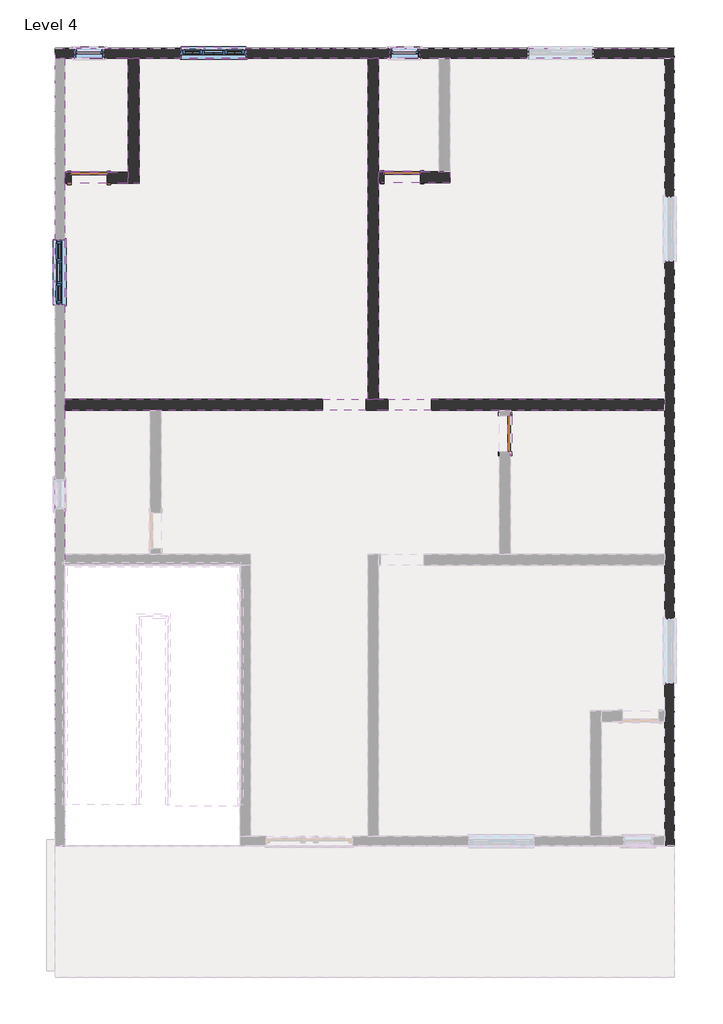
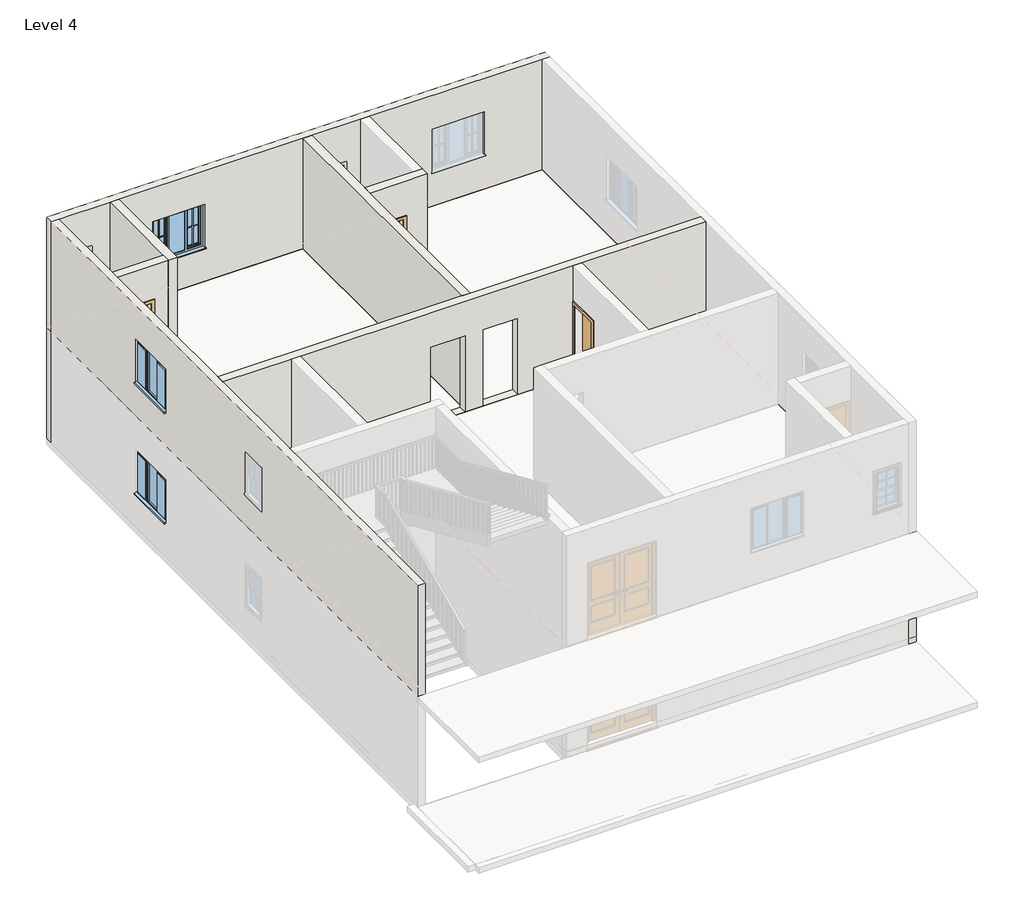
# One storey, part 2 of 5: 20 walls, 12 windows, 9 doors.
"""IFC4 building model written with IfcOpenShell, lengths in millimetres."""

from ifc_helpers import new_model, si_unit, frame, origin, place, context, project, spatial, polyline, outline, extrude, faceted_brep, transform, mapped, element, save
from components import door_85036156, window_679d2811, windows_tpl_w_glazing_cross_bars_1360x1210mm_0306471f

model = new_model("IFC4")

# Units and contexts
model_context = context("Model", 3, world=origin())
ifc_project = project(units=[si_unit("LENGTHUNIT", "METRE", prefix="MILLI")], contexts=[model_context])

# Site, building, storey
site = spatial("IfcSite", under=ifc_project)
building = spatial("IfcBuilding", under=site)
storey = spatial("IfcBuildingStorey", under=building, Name="Level 4", Elevation=9144.0)

# Doors
placement = place(None, origin())
door_shape = door_85036156(model_context)
element("IfcDoor", 1, ObjectType="Single-Flush : 30\" x 80\"", at=placement, inside=storey, context=model_context, shape_type="MappedRepresentation", body=[
    mapped(door_shape, transform((-7046.4415084, 6189.6935985, 9144.0), x_axis=(-1.0, 0.0, 0.0), y_axis=(0.0, -1.0, 0.0), z_axis=(0.0, 0.0, 1.0))),
])
element("IfcDoor", 2, ObjectType="Single-Flush : 30\" x 80\"", at=placement, inside=storey, context=model_context, shape_type="MappedRepresentation", body=[
    mapped(door_shape, transform((-467.8415084, 6203.2000968, 9144.0), x_axis=(-1.0, 0.0, 0.0), y_axis=(0.0, -1.0, 0.0), z_axis=(0.0, 0.0, 1.0))),
])
element("IfcDoor", 3, ObjectType="Single-Flush : 30\" x 80\"", at=placement, inside=storey, context=model_context, shape_type="MappedRepresentation", body=[
    mapped(door_shape, transform((1691.1584916, 817.5935985, 9144.0), x_axis=(0.0, 1.0, 0.0), y_axis=(-1.0, 0.0, 0.0), z_axis=(0.0, 0.0, 1.0))),
])
element("IfcDoor", 4, ObjectType="Single-Flush : 30\" x 80\"", at=placement, inside=storey, context=model_context, shape_type="MappedRepresentation", body=[
    mapped(door_shape, transform((-7046.4415084, 6189.6935985, 9144.0), x_axis=(-1.0, 0.0, 0.0), y_axis=(0.0, -1.0, 0.0), z_axis=(0.0, 0.0, 1.0))),
])
element("IfcDoor", 5, ObjectType="Single-Flush : 30\" x 80\"", at=placement, inside=storey, context=model_context, shape_type="MappedRepresentation", body=[
    mapped(door_shape, transform((-467.8415084, 6203.2000968, 9144.0), x_axis=(-1.0, 0.0, 0.0), y_axis=(0.0, -1.0, 0.0), z_axis=(0.0, 0.0, 1.0))),
])
element("IfcDoor", 6, ObjectType="Single-Flush : 30\" x 80\"", at=placement, inside=storey, context=model_context, shape_type="MappedRepresentation", body=[
    mapped(door_shape, transform((1691.1584916, 817.5935985, 9144.0), x_axis=(0.0, 1.0, 0.0), y_axis=(-1.0, 0.0, 0.0), z_axis=(0.0, 0.0, 1.0))),
])
element("IfcDoor", 7, ObjectType="Single-Flush : 30\" x 80\"", at=placement, inside=storey, context=model_context, shape_type="MappedRepresentation", body=[
    mapped(door_shape, transform((-7046.4415084, 6189.6935985, 12192.0), x_axis=(-1.0, 0.0, 0.0), y_axis=(0.0, -1.0, 0.0), z_axis=(0.0, 0.0, 1.0))),
])
element("IfcDoor", 8, ObjectType="Single-Flush : 30\" x 80\"", at=placement, inside=storey, context=model_context, shape_type="MappedRepresentation", body=[
    mapped(door_shape, transform((-467.8415084, 6203.2000968, 12192.0), x_axis=(-1.0, 0.0, 0.0), y_axis=(0.0, -1.0, 0.0), z_axis=(0.0, 0.0, 1.0))),
])
element("IfcDoor", 9, ObjectType="Single-Flush : 30\" x 80\"", at=placement, inside=storey, context=model_context, shape_type="MappedRepresentation", body=[
    mapped(door_shape, transform((1691.1584916, 817.5935985, 12192.0), x_axis=(0.0, 1.0, 0.0), y_axis=(-1.0, 0.0, 0.0), z_axis=(0.0, 0.0, 1.0))),
])

# Walls
element("IfcWall", 10, ObjectType="Generic - 4.5\"", at=placement, inside=storey, context=model_context, shape_type="Brep", body=[
    faceted_brep([(-1232.0415084, 1312.8935985, 11254.0), (-1232.0415084, 1312.8935985, 9144.0), (-770.4415084, 1312.8935985, 9144.0), (-770.4415084, 1312.8935985, 11254.0), (139.5584916, 1312.8935985, 11254.0), (139.5584916, 1312.8935985, 9144.0), (1576.8584916, 1312.8935985, 9144.0), (1805.4584916, 1312.8935985, 9144.0), (5043.9584916, 1312.8935985, 9144.0), (5043.9584916, 1312.8935985, 12192.0), (1805.4584916, 1312.8935985, 12192.0), (1576.8584916, 1312.8935985, 12192.0), (-5535.1415084, 1312.8935985, 12192.0), (-5763.7415084, 1312.8935985, 12192.0), (-7554.4415084, 1312.8935985, 12192.0), (-7554.4415084, 1312.8935985, 9144.0), (-5763.7415084, 1312.8935985, 9144.0), (-5535.1415084, 1312.8935985, 9144.0), (-2142.0415084, 1312.8935985, 9144.0), (-2142.0415084, 1312.8935985, 11254.0), (-770.4415084, 1541.4935985, 9144.0), (-963.1415084, 1541.4935985, 9144.0), (-1191.7415084, 1541.4935985, 9144.0), (-1232.0415084, 1541.4935985, 9144.0), (-1232.0415084, 1541.4935985, 11254.0), (-2142.0415084, 1541.4935985, 11254.0), (-2142.0415084, 1541.4935985, 9144.0), (-7554.4415084, 1541.4935985, 9144.0), (-7554.4415084, 1541.4935985, 12192.0), (-1191.7415084, 1541.4935985, 12192.0), (-963.1415084, 1541.4935985, 12192.0), (5043.9584916, 1541.4935985, 12192.0), (5043.9584916, 1541.4935985, 9144.0), (139.5584916, 1541.4935985, 9144.0), (139.5584916, 1541.4935985, 11254.0), (-770.4415084, 1541.4935985, 11254.0)], [[[0, 1, 2, 3, 4, 5, 6, 7, 8, 9, 10, 11, 12, 13, 14, 15, 16, 17, 18, 19]], [[20, 21, 22, 23, 24, 25, 26, 27, 28, 29, 30, 31, 32, 33, 34, 35]], [[33, 32, 8, 7, 6, 5]], [[2, 1, 23, 22, 21, 20]], [[18, 17, 16, 15, 27, 26]], [[14, 13, 12, 11, 10, 9, 31, 30, 29, 28]], [[9, 8, 32, 31]], [[15, 14, 28, 27]], [[5, 4, 34, 33]], [[3, 2, 20, 35]], [[4, 3, 35, 34]], [[26, 25, 19, 18]], [[24, 23, 1, 0]], [[25, 24, 0, 19]]]),
])
element("IfcWall", 11, ObjectType="Generic - 4.5\"", at=placement, inside=storey, context=model_context, shape_type="Brep", body=[
    faceted_brep([(-1191.7415084, 8704.2935985, 9144.0), (-1191.7415084, 1541.4935985, 9144.0), (-1191.7415084, 1541.4935985, 12192.0), (-1191.7415084, 8704.2935985, 12192.0), (-963.1415084, 8704.2935985, 9144.0), (-963.1415084, 8704.2935985, 12192.0), (-963.1415084, 6317.5000968, 12192.0), (-963.1415084, 6088.9000968, 12192.0), (-963.1415084, 1541.4935985, 12192.0), (-963.1415084, 1541.4935985, 9144.0), (-963.1415084, 6088.9000968, 9144.0), (-963.1415084, 6317.5000968, 9144.0)], [[[0, 1, 2, 3]], [[4, 5, 6, 7, 8, 9, 10, 11]], [[1, 0, 4, 11, 10, 9]], [[3, 2, 8, 7, 6, 5]], [[0, 3, 5, 4]], [[2, 1, 9, 8]]]),
])
element("IfcWall", 12, ObjectType="Generic - 4.5\"", at=placement, inside=storey, context=model_context, shape_type="Brep", body=[
    faceted_brep([(-6220.9415084, 8704.2935985, 9144.0), (-6220.9415084, 6303.9935985, 9144.0), (-6220.9415084, 6075.3935985, 9144.0), (-6220.9415084, 6075.3935985, 12192.0), (-6220.9415084, 6303.9935985, 12192.0), (-6220.9415084, 8704.2935985, 12192.0), (-5992.3415084, 8704.2935985, 9144.0), (-5992.3415084, 8704.2935985, 12192.0), (-5992.3415084, 6075.3935985, 12192.0), (-5992.3415084, 6075.3935985, 9144.0)], [[[0, 1, 2, 3, 4, 5]], [[6, 7, 8, 9]], [[2, 1, 0, 6, 9]], [[5, 4, 3, 8, 7]], [[0, 5, 7, 6]], [[3, 2, 9, 8]]]),
])
element("IfcWall", 13, ObjectType="Generic - 4.5\"", at=placement, inside=storey, context=model_context, shape_type="SweptSolid", body=[
    extrude(outline(polyline([(9144.0, -7554.4415084), (9144.0, -7427.4415084), (11176.0, -7427.4415084), (11176.0, -6665.4415084), (9144.0, -6665.4415084), (9144.0, -6220.9415084), (12192.0, -6220.9415084), (12192.0, -7554.4415084), (9144.0, -7554.4415084)])), frame((0.0, 6075.3935985, 0.0), z_axis=(0.0, 1.0, 0.0), x_axis=(0.0, 0.0, 1.0)), (0.0, 0.0, 1.0), 228.6),
])
element("IfcWall", 14, ObjectType="Generic - 4.5\"", at=placement, inside=storey, context=model_context, shape_type="Brep", body=[
    faceted_brep([(-963.1415084, 6088.9000968, 9144.0), (-848.8415084, 6088.9000968, 9144.0), (-848.8415084, 6088.9000968, 11176.0), (-86.8415084, 6088.9000968, 11176.0), (-86.8415084, 6088.9000968, 9144.0), (535.4584916, 6088.9000968, 9144.0), (535.4584916, 6088.9000968, 12192.0), (-963.1415084, 6088.9000968, 12192.0), (-848.8415084, 6317.5000968, 11176.0), (-848.8415084, 6317.5000968, 9144.0), (-963.1415084, 6317.5000968, 9144.0), (-963.1415084, 6317.5000968, 12192.0), (306.8584916, 6317.5000968, 12192.0), (535.4584916, 6317.5000968, 12192.0), (535.4584916, 6317.5000968, 9144.0), (306.8584916, 6317.5000968, 9144.0), (-86.8415084, 6317.5000968, 9144.0), (-86.8415084, 6317.5000968, 11176.0)], [[[0, 1, 2, 3, 4, 5, 6, 7]], [[8, 9, 10, 11, 12, 13, 14, 15, 16, 17]], [[10, 9, 1, 0]], [[16, 15, 14, 5, 4]], [[7, 6, 13, 12, 11]], [[0, 7, 11, 10]], [[6, 5, 14, 13]], [[2, 1, 9, 8]], [[3, 2, 8, 17]], [[4, 3, 17, 16]]]),
])
element("IfcWall", 15, ObjectType="Generic - 4.5\"", at=placement, inside=storey, context=model_context, shape_type="Brep", body=[
    faceted_brep([(-1232.0415084, 1312.8935985, 11254.0), (-1232.0415084, 1312.8935985, 9144.0), (-770.4415084, 1312.8935985, 9144.0), (-770.4415084, 1312.8935985, 11254.0), (139.5584916, 1312.8935985, 11254.0), (139.5584916, 1312.8935985, 9144.0), (1576.8584916, 1312.8935985, 9144.0), (1805.4584916, 1312.8935985, 9144.0), (5043.9584916, 1312.8935985, 9144.0), (5043.9584916, 1312.8935985, 12192.0), (1805.4584916, 1312.8935985, 12192.0), (1576.8584916, 1312.8935985, 12192.0), (-5535.1415084, 1312.8935985, 12192.0), (-5763.7415084, 1312.8935985, 12192.0), (-7554.4415084, 1312.8935985, 12192.0), (-7554.4415084, 1312.8935985, 9144.0), (-5763.7415084, 1312.8935985, 9144.0), (-5535.1415084, 1312.8935985, 9144.0), (-2142.0415084, 1312.8935985, 9144.0), (-2142.0415084, 1312.8935985, 11254.0), (-770.4415084, 1541.4935985, 9144.0), (-963.1415084, 1541.4935985, 9144.0), (-1191.7415084, 1541.4935985, 9144.0), (-1232.0415084, 1541.4935985, 9144.0), (-1232.0415084, 1541.4935985, 11254.0), (-2142.0415084, 1541.4935985, 11254.0), (-2142.0415084, 1541.4935985, 9144.0), (-7554.4415084, 1541.4935985, 9144.0), (-7554.4415084, 1541.4935985, 12192.0), (-1191.7415084, 1541.4935985, 12192.0), (-963.1415084, 1541.4935985, 12192.0), (5043.9584916, 1541.4935985, 12192.0), (5043.9584916, 1541.4935985, 9144.0), (139.5584916, 1541.4935985, 9144.0), (139.5584916, 1541.4935985, 11254.0), (-770.4415084, 1541.4935985, 11254.0)], [[[0, 1, 2, 3, 4, 5, 6, 7, 8, 9, 10, 11, 12, 13, 14, 15, 16, 17, 18, 19]], [[20, 21, 22, 23, 24, 25, 26, 27, 28, 29, 30, 31, 32, 33, 34, 35]], [[33, 32, 8, 7, 6, 5]], [[2, 1, 23, 22, 21, 20]], [[18, 17, 16, 15, 27, 26]], [[14, 13, 12, 11, 10, 9, 31, 30, 29, 28]], [[9, 8, 32, 31]], [[15, 14, 28, 27]], [[5, 4, 34, 33]], [[3, 2, 20, 35]], [[4, 3, 35, 34]], [[26, 25, 19, 18]], [[24, 23, 1, 0]], [[25, 24, 0, 19]]]),
])
element("IfcWall", 16, ObjectType="Generic - 4.5\"", at=placement, inside=storey, context=model_context, shape_type="Brep", body=[
    faceted_brep([(-1191.7415084, 8704.2935985, 9144.0), (-1191.7415084, 1541.4935985, 9144.0), (-1191.7415084, 1541.4935985, 12192.0), (-1191.7415084, 8704.2935985, 12192.0), (-963.1415084, 8704.2935985, 9144.0), (-963.1415084, 8704.2935985, 12192.0), (-963.1415084, 6317.5000968, 12192.0), (-963.1415084, 6088.9000968, 12192.0), (-963.1415084, 1541.4935985, 12192.0), (-963.1415084, 1541.4935985, 9144.0), (-963.1415084, 6088.9000968, 9144.0), (-963.1415084, 6317.5000968, 9144.0)], [[[0, 1, 2, 3]], [[4, 5, 6, 7, 8, 9, 10, 11]], [[1, 0, 4, 11, 10, 9]], [[3, 2, 8, 7, 6, 5]], [[0, 3, 5, 4]], [[2, 1, 9, 8]]]),
])
element("IfcWall", 17, ObjectType="Generic - 4.5\"", at=placement, inside=storey, context=model_context, shape_type="SweptSolid", body=[
    extrude(outline(polyline([(-6220.9415084, 6303.9935985), (-6220.9415084, 8704.2935985), (-5992.3415084, 8704.2935985), (-5992.3415084, 6303.9935985), (-6220.9415084, 6303.9935985)])), frame((0.0, 0.0, 9144.0), z_axis=(0.0, 0.0, 1.0), x_axis=(1.0, 0.0, 0.0)), (0.0, 0.0, 1.0), 3048.0),
])
element("IfcWall", 18, ObjectType="Generic - 4.5\"", at=placement, inside=storey, context=model_context, shape_type="SweptSolid", body=[
    extrude(outline(polyline([(9144.0, -7554.4415084), (9144.0, -7427.4415084), (11176.0, -7427.4415084), (11176.0, -6665.4415084), (9144.0, -6665.4415084), (9144.0, -6220.9415084), (12192.0, -6220.9415084), (12192.0, -7554.4415084), (9144.0, -7554.4415084)])), frame((0.0, 6075.3935985, 0.0), z_axis=(0.0, 1.0, 0.0), x_axis=(0.0, 0.0, 1.0)), (0.0, 0.0, 1.0), 228.6),
])
element("IfcWall", 19, ObjectType="Generic - 4.5\"", at=placement, inside=storey, context=model_context, shape_type="SweptSolid", body=[
    extrude(outline(polyline([(9144.0, -963.1415084), (9144.0, -848.8415084), (11176.0, -848.8415084), (11176.0, -86.8415084), (9144.0, -86.8415084), (9144.0, 306.8584916), (12192.0, 306.8584916), (12192.0, -963.1415084), (9144.0, -963.1415084)])), frame((0.0, 6088.9000968, 0.0), z_axis=(0.0, 1.0, 0.0), x_axis=(0.0, 0.0, 1.0)), (0.0, 0.0, 1.0), 228.6),
])
element("IfcWall", 20, ObjectType="Generic - 4.5\"", at=placement, inside=storey, context=model_context, shape_type="Brep", body=[
    faceted_brep([(-1232.0415084, 1312.8935985, 14302.0), (-1232.0415084, 1312.8935985, 12192.0), (-770.4415084, 1312.8935985, 12192.0), (-770.4415084, 1312.8935985, 14302.0), (139.5584916, 1312.8935985, 14302.0), (139.5584916, 1312.8935985, 12192.0), (1576.8584916, 1312.8935985, 12192.0), (1805.4584916, 1312.8935985, 12192.0), (5043.9584916, 1312.8935985, 12192.0), (5043.9584916, 1312.8935985, 15240.0), (1805.4584916, 1312.8935985, 15240.0), (1576.8584916, 1312.8935985, 15240.0), (-5535.1415084, 1312.8935985, 15240.0), (-5763.7415084, 1312.8935985, 15240.0), (-7554.4415084, 1312.8935985, 15240.0), (-7554.4415084, 1312.8935985, 12192.0), (-5763.7415084, 1312.8935985, 12192.0), (-5535.1415084, 1312.8935985, 12192.0), (-2142.0415084, 1312.8935985, 12192.0), (-2142.0415084, 1312.8935985, 14302.0), (-770.4415084, 1541.4935985, 12192.0), (-963.1415084, 1541.4935985, 12192.0), (-1191.7415084, 1541.4935985, 12192.0), (-1232.0415084, 1541.4935985, 12192.0), (-1232.0415084, 1541.4935985, 14302.0), (-2142.0415084, 1541.4935985, 14302.0), (-2142.0415084, 1541.4935985, 12192.0), (-7554.4415084, 1541.4935985, 12192.0), (-7554.4415084, 1541.4935985, 15240.0), (-1191.7415084, 1541.4935985, 15240.0), (-963.1415084, 1541.4935985, 15240.0), (5043.9584916, 1541.4935985, 15240.0), (5043.9584916, 1541.4935985, 12192.0), (139.5584916, 1541.4935985, 12192.0), (139.5584916, 1541.4935985, 14302.0), (-770.4415084, 1541.4935985, 14302.0)], [[[0, 1, 2, 3, 4, 5, 6, 7, 8, 9, 10, 11, 12, 13, 14, 15, 16, 17, 18, 19]], [[20, 21, 22, 23, 24, 25, 26, 27, 28, 29, 30, 31, 32, 33, 34, 35]], [[33, 32, 8, 7, 6, 5]], [[2, 1, 23, 22, 21, 20]], [[18, 17, 16, 15, 27, 26]], [[14, 13, 12, 11, 10, 9, 31, 30, 29, 28]], [[9, 8, 32, 31]], [[15, 14, 28, 27]], [[5, 4, 34, 33]], [[3, 2, 20, 35]], [[4, 3, 35, 34]], [[26, 25, 19, 18]], [[24, 23, 1, 0]], [[25, 24, 0, 19]]]),
])
element("IfcWall", 21, ObjectType="Generic - 4.5\"", at=placement, inside=storey, context=model_context, shape_type="Brep", body=[
    faceted_brep([(-1191.7415084, 8704.2935985, 12192.0), (-1191.7415084, 1541.4935985, 12192.0), (-1191.7415084, 1541.4935985, 15240.0), (-1191.7415084, 8704.2935985, 15240.0), (-963.1415084, 8704.2935985, 12192.0), (-963.1415084, 8704.2935985, 15240.0), (-963.1415084, 6317.5000968, 15240.0), (-963.1415084, 6088.9000968, 15240.0), (-963.1415084, 1541.4935985, 15240.0), (-963.1415084, 1541.4935985, 12192.0), (-963.1415084, 6088.9000968, 12192.0), (-963.1415084, 6317.5000968, 12192.0)], [[[0, 1, 2, 3]], [[4, 5, 6, 7, 8, 9, 10, 11]], [[1, 0, 4, 11, 10, 9]], [[3, 2, 8, 7, 6, 5]], [[0, 3, 5, 4]], [[2, 1, 9, 8]]]),
])
element("IfcWall", 22, ObjectType="Generic - 4.5\"", at=placement, inside=storey, context=model_context, shape_type="Brep", body=[
    faceted_brep([(-6220.9415084, 8704.2935985, 12192.0), (-6220.9415084, 6303.9935985, 12192.0), (-6220.9415084, 6075.3935985, 12192.0), (-6220.9415084, 6075.3935985, 15240.0), (-6220.9415084, 6303.9935985, 15240.0), (-6220.9415084, 8704.2935985, 15240.0), (-5992.3415084, 8704.2935985, 12192.0), (-5992.3415084, 8704.2935985, 15240.0), (-5992.3415084, 6075.3935985, 15240.0), (-5992.3415084, 6075.3935985, 12192.0)], [[[0, 1, 2, 3, 4, 5]], [[6, 7, 8, 9]], [[2, 1, 0, 6, 9]], [[5, 4, 3, 8, 7]], [[0, 5, 7, 6]], [[3, 2, 9, 8]]]),
])
element("IfcWall", 23, ObjectType="Generic - 4.5\"", at=placement, inside=storey, context=model_context, shape_type="SweptSolid", body=[
    extrude(outline(polyline([(12192.0, -7554.4415084), (12192.0, -7427.4415084), (14224.0, -7427.4415084), (14224.0, -6665.4415084), (12192.0, -6665.4415084), (12192.0, -6220.9415084), (15240.0, -6220.9415084), (15240.0, -7554.4415084), (12192.0, -7554.4415084)])), frame((0.0, 6075.3935985, 0.0), z_axis=(0.0, 1.0, 0.0), x_axis=(0.0, 0.0, 1.0)), (0.0, 0.0, 1.0), 228.6),
])
element("IfcWall", 24, ObjectType="Generic - 4.5\"", at=placement, inside=storey, context=model_context, shape_type="Brep", body=[
    faceted_brep([(-963.1415084, 6088.9000968, 12192.0), (-848.8415084, 6088.9000968, 12192.0), (-848.8415084, 6088.9000968, 14224.0), (-86.8415084, 6088.9000968, 14224.0), (-86.8415084, 6088.9000968, 12192.0), (535.4584916, 6088.9000968, 12192.0), (535.4584916, 6088.9000968, 15240.0), (-963.1415084, 6088.9000968, 15240.0), (-848.8415084, 6317.5000968, 14224.0), (-848.8415084, 6317.5000968, 12192.0), (-963.1415084, 6317.5000968, 12192.0), (-963.1415084, 6317.5000968, 15240.0), (306.8584916, 6317.5000968, 15240.0), (535.4584916, 6317.5000968, 15240.0), (535.4584916, 6317.5000968, 12192.0), (306.8584916, 6317.5000968, 12192.0), (-86.8415084, 6317.5000968, 12192.0), (-86.8415084, 6317.5000968, 14224.0)], [[[0, 1, 2, 3, 4, 5, 6, 7]], [[8, 9, 10, 11, 12, 13, 14, 15, 16, 17]], [[10, 9, 1, 0]], [[16, 15, 14, 5, 4]], [[7, 6, 13, 12, 11]], [[0, 7, 11, 10]], [[6, 5, 14, 13]], [[2, 1, 9, 8]], [[3, 2, 8, 17]], [[4, 3, 17, 16]]]),
])
element("IfcWall", 25, ObjectType="Generic - 9\"", at=placement, inside=storey, context=model_context, shape_type="Brep", body=[
    faceted_brep([(-7757.6415084, 8704.2935985, 9144.0), (-7554.4415084, 8704.2935985, 9144.0), (-6220.9415084, 8704.2935985, 9144.0), (-5992.3415084, 8704.2935985, 9144.0), (-1191.7415084, 8704.2935985, 9144.0), (-963.1415084, 8704.2935985, 9144.0), (306.8584916, 8704.2935985, 9144.0), (535.4584916, 8704.2935985, 9144.0), (5043.9584916, 8704.2935985, 9144.0), (5247.1584916, 8704.2935985, 9144.0), (5247.1584916, 8704.2935985, 12192.0), (5043.9584916, 8704.2935985, 12192.0), (535.4584916, 8704.2935985, 12192.0), (306.8584916, 8704.2935985, 12192.0), (-963.1415084, 8704.2935985, 12192.0), (-1191.7415084, 8704.2935985, 12192.0), (-5992.3415084, 8704.2935985, 12192.0), (-6220.9415084, 8704.2935985, 12192.0), (-7554.4415084, 8704.2935985, 12192.0), (-7757.6415084, 8704.2935985, 12192.0), (2179.5584916, 8704.2935985, 11268.4), (3539.5584916, 8704.2935985, 11268.4), (3539.5584916, 8704.2935985, 10058.4), (2179.5584916, 8704.2935985, 10058.4), (-5110.2415084, 8704.2935985, 11268.4), (-3750.2415084, 8704.2935985, 11268.4), (-3750.2415084, 8704.2935985, 10058.4), (-5110.2415084, 8704.2935985, 10058.4), (-7351.2415084, 8704.2935985, 11125.2), (-6741.6415084, 8704.2935985, 11125.2), (-6741.6415084, 8704.2935985, 10058.4), (-7351.2415084, 8704.2935985, 10058.4), (-721.8415084, 8704.2935985, 11125.2), (-112.2415084, 8704.2935985, 11125.2), (-112.2415084, 8704.2935985, 10058.4), (-721.8415084, 8704.2935985, 10058.4), (-7757.6415084, 8907.4935985, 9144.0), (-7757.6415084, 8907.4935985, 12192.0), (5247.1584916, 8907.4935985, 12192.0), (5247.1584916, 8907.4935985, 9144.0), (2179.5584916, 8907.4935985, 11268.4), (2179.5584916, 8907.4935985, 10058.4), (3539.5584916, 8907.4935985, 10058.4), (3539.5584916, 8907.4935985, 11268.4), (-5110.2415084, 8907.4935985, 11268.4), (-5110.2415084, 8907.4935985, 10058.4), (-3750.2415084, 8907.4935985, 10058.4), (-3750.2415084, 8907.4935985, 11268.4), (-7351.2415084, 8907.4935985, 11125.2), (-7351.2415084, 8907.4935985, 10058.4), (-6741.6415084, 8907.4935985, 10058.4), (-6741.6415084, 8907.4935985, 11125.2), (-721.8415084, 8907.4935985, 11125.2), (-721.8415084, 8907.4935985, 10058.4), (-112.2415084, 8907.4935985, 10058.4), (-112.2415084, 8907.4935985, 11125.2)], [[[0, 1, 2, 3, 4, 5, 6, 7, 8, 9, 10, 11, 12, 13, 14, 15, 16, 17, 18, 19], [20, 21, 22, 23], [24, 25, 26, 27], [28, 29, 30, 31], [32, 33, 34, 35]], [[36, 37, 38, 39], [40, 41, 42, 43], [44, 45, 46, 47], [48, 49, 50, 51], [52, 53, 54, 55]], [[9, 8, 7, 6, 5, 4, 3, 2, 1, 0, 36, 39]], [[19, 18, 17, 16, 15, 14, 13, 12, 11, 10, 38, 37]], [[10, 9, 39, 38]], [[41, 40, 20, 23]], [[42, 41, 23, 22]], [[43, 42, 22, 21]], [[40, 43, 21, 20]], [[45, 44, 24, 27]], [[46, 45, 27, 26]], [[47, 46, 26, 25]], [[44, 47, 25, 24]], [[49, 48, 28, 31]], [[50, 49, 31, 30]], [[51, 50, 30, 29]], [[48, 51, 29, 28]], [[53, 52, 32, 35]], [[54, 53, 35, 34]], [[55, 54, 34, 33]], [[52, 55, 33, 32]], [[0, 19, 37, 36]]]),
])
element("IfcWall", 26, ObjectType="Generic - 9\"", at=placement, inside=storey, context=model_context, shape_type="Brep", body=[
    faceted_brep([(5043.9584916, 8704.2935985, 9144.0), (5043.9584916, 1541.4935985, 9144.0), (5043.9584916, 1312.8935985, 9144.0), (5043.9584916, -1712.5217109, 9144.0), (5043.9584916, -1941.1217109, 9144.0), (5043.9584916, -4999.0064015, 9144.0), (5043.9584916, -5227.6064015, 9144.0), (5043.9584916, -7627.9064015, 9144.0), (5043.9584916, -7831.1064015, 9144.0), (5043.9584916, -7831.1064015, 12192.0), (5043.9584916, -7627.9064015, 12192.0), (5043.9584916, -5227.6064015, 12192.0), (5043.9584916, -4999.0064015, 12192.0), (5043.9584916, -1941.1217109, 12192.0), (5043.9584916, -1712.5217109, 12192.0), (5043.9584916, 1312.8935985, 12192.0), (5043.9584916, 1541.4935985, 12192.0), (5043.9584916, 8704.2935985, 12192.0), (5043.9584916, 5796.5435985, 11268.4), (5043.9584916, 4436.5435985, 11268.4), (5043.9584916, 4436.5435985, 10058.4), (5043.9584916, 5796.5435985, 10058.4), (5043.9584916, -3061.7064015, 11268.4), (5043.9584916, -4421.7064015, 11268.4), (5043.9584916, -4421.7064015, 10058.4), (5043.9584916, -3061.7064015, 10058.4), (5247.1584916, 8704.2935985, 9144.0), (5247.1584916, 8704.2935985, 12192.0), (5247.1584916, -7831.1064015, 12192.0), (5247.1584916, -7831.1064015, 9144.0), (5247.1584916, 5796.5435985, 11268.4), (5247.1584916, 5796.5435985, 10058.4), (5247.1584916, 4436.5435985, 10058.4), (5247.1584916, 4436.5435985, 11268.4), (5247.1584916, -3061.7064015, 11268.4), (5247.1584916, -3061.7064015, 10058.4), (5247.1584916, -4421.7064015, 10058.4), (5247.1584916, -4421.7064015, 11268.4)], [[[0, 1, 2, 3, 4, 5, 6, 7, 8, 9, 10, 11, 12, 13, 14, 15, 16, 17], [18, 19, 20, 21], [22, 23, 24, 25]], [[26, 27, 28, 29], [30, 31, 32, 33], [34, 35, 36, 37]], [[8, 7, 6, 5, 4, 3, 2, 1, 0, 26, 29]], [[17, 16, 15, 14, 13, 12, 11, 10, 9, 28, 27]], [[31, 30, 18, 21]], [[32, 31, 21, 20]], [[33, 32, 20, 19]], [[30, 33, 19, 18]], [[35, 34, 22, 25]], [[36, 35, 25, 24]], [[37, 36, 24, 23]], [[34, 37, 23, 22]], [[0, 17, 27, 26]], [[9, 8, 29, 28]]]),
])
element("IfcWall", 27, ObjectType="Generic - 9\"", at=placement, inside=storey, context=model_context, shape_type="Brep", body=[
    faceted_brep([(-7554.4415084, 8704.2935985, 9144.0), (-6220.9415084, 8704.2935985, 9144.0), (-5992.3415084, 8704.2935985, 9144.0), (-1191.7415084, 8704.2935985, 9144.0), (-963.1415084, 8704.2935985, 9144.0), (306.8584916, 8704.2935985, 9144.0), (535.4584916, 8704.2935985, 9144.0), (5043.9584916, 8704.2935985, 9144.0), (5043.9584916, 8704.2935985, 12192.0), (535.4584916, 8704.2935985, 12192.0), (306.8584916, 8704.2935985, 12192.0), (-963.1415084, 8704.2935985, 12192.0), (-1191.7415084, 8704.2935985, 12192.0), (-5992.3415084, 8704.2935985, 12192.0), (-6220.9415084, 8704.2935985, 12192.0), (-7554.4415084, 8704.2935985, 12192.0), (2179.5584916, 8704.2935985, 11268.4), (3539.5584916, 8704.2935985, 11268.4), (3539.5584916, 8704.2935985, 10058.4), (2179.5584916, 8704.2935985, 10058.4), (-5110.2415084, 8704.2935985, 11268.4), (-3750.2415084, 8704.2935985, 11268.4), (-3750.2415084, 8704.2935985, 10058.4), (-5110.2415084, 8704.2935985, 10058.4), (-7351.2415084, 8704.2935985, 11125.2), (-6741.6415084, 8704.2935985, 11125.2), (-6741.6415084, 8704.2935985, 10058.4), (-7351.2415084, 8704.2935985, 10058.4), (-721.8415084, 8704.2935985, 11125.2), (-112.2415084, 8704.2935985, 11125.2), (-112.2415084, 8704.2935985, 10058.4), (-721.8415084, 8704.2935985, 10058.4), (-7554.4415084, 8907.4935985, 9144.0), (-7554.4415084, 8907.4935985, 12192.0), (5043.9584916, 8907.4935985, 12192.0), (5043.9584916, 8907.4935985, 9144.0), (2179.5584916, 8907.4935985, 11268.4), (2179.5584916, 8907.4935985, 10058.4), (3539.5584916, 8907.4935985, 10058.4), (3539.5584916, 8907.4935985, 11268.4), (-5110.2415084, 8907.4935985, 11268.4), (-5110.2415084, 8907.4935985, 10058.4), (-3750.2415084, 8907.4935985, 10058.4), (-3750.2415084, 8907.4935985, 11268.4), (-7351.2415084, 8907.4935985, 11125.2), (-7351.2415084, 8907.4935985, 10058.4), (-6741.6415084, 8907.4935985, 10058.4), (-6741.6415084, 8907.4935985, 11125.2), (-721.8415084, 8907.4935985, 11125.2), (-721.8415084, 8907.4935985, 10058.4), (-112.2415084, 8907.4935985, 10058.4), (-112.2415084, 8907.4935985, 11125.2)], [[[0, 1, 2, 3, 4, 5, 6, 7, 8, 9, 10, 11, 12, 13, 14, 15], [16, 17, 18, 19], [20, 21, 22, 23], [24, 25, 26, 27], [28, 29, 30, 31]], [[32, 33, 34, 35], [36, 37, 38, 39], [40, 41, 42, 43], [44, 45, 46, 47], [48, 49, 50, 51]], [[7, 6, 5, 4, 3, 2, 1, 0, 32, 35]], [[15, 14, 13, 12, 11, 10, 9, 8, 34, 33]], [[37, 36, 16, 19]], [[38, 37, 19, 18]], [[39, 38, 18, 17]], [[36, 39, 17, 16]], [[41, 40, 20, 23]], [[42, 41, 23, 22]], [[43, 42, 22, 21]], [[40, 43, 21, 20]], [[45, 44, 24, 27]], [[46, 45, 27, 26]], [[47, 46, 26, 25]], [[44, 47, 25, 24]], [[49, 48, 28, 31]], [[50, 49, 31, 30]], [[51, 50, 30, 29]], [[48, 51, 29, 28]], [[8, 7, 35, 34]], [[0, 15, 33, 32]]]),
])
element("IfcWall", 28, ObjectType="Generic - 9\"", at=placement, inside=storey, context=model_context, shape_type="Brep", body=[
    faceted_brep([(-7757.6415084, 8704.2935985, 12192.0), (-7554.4415084, 8704.2935985, 12192.0), (-6220.9415084, 8704.2935985, 12192.0), (-5992.3415084, 8704.2935985, 12192.0), (-1191.7415084, 8704.2935985, 12192.0), (-963.1415084, 8704.2935985, 12192.0), (306.8584916, 8704.2935985, 12192.0), (535.4584916, 8704.2935985, 12192.0), (5043.9584916, 8704.2935985, 12192.0), (5247.1584916, 8704.2935985, 12192.0), (5247.1584916, 8704.2935985, 15240.0), (5043.9584916, 8704.2935985, 15240.0), (535.4584916, 8704.2935985, 15240.0), (306.8584916, 8704.2935985, 15240.0), (-963.1415084, 8704.2935985, 15240.0), (-1191.7415084, 8704.2935985, 15240.0), (-5992.3415084, 8704.2935985, 15240.0), (-6220.9415084, 8704.2935985, 15240.0), (-7554.4415084, 8704.2935985, 15240.0), (-7757.6415084, 8704.2935985, 15240.0), (2179.5584916, 8704.2935985, 14316.4), (3539.5584916, 8704.2935985, 14316.4), (3539.5584916, 8704.2935985, 13106.4), (2179.5584916, 8704.2935985, 13106.4), (-5110.2415084, 8704.2935985, 14316.4), (-3750.2415084, 8704.2935985, 14316.4), (-3750.2415084, 8704.2935985, 13106.4), (-5110.2415084, 8704.2935985, 13106.4), (-7351.2415084, 8704.2935985, 14173.2), (-6741.6415084, 8704.2935985, 14173.2), (-6741.6415084, 8704.2935985, 13106.4), (-7351.2415084, 8704.2935985, 13106.4), (-721.8415084, 8704.2935985, 14173.2), (-112.2415084, 8704.2935985, 14173.2), (-112.2415084, 8704.2935985, 13106.4), (-721.8415084, 8704.2935985, 13106.4), (-7757.6415084, 8907.4935985, 12192.0), (-7757.6415084, 8907.4935985, 15240.0), (5247.1584916, 8907.4935985, 15240.0), (5247.1584916, 8907.4935985, 12192.0), (2179.5584916, 8907.4935985, 14316.4), (2179.5584916, 8907.4935985, 13106.4), (3539.5584916, 8907.4935985, 13106.4), (3539.5584916, 8907.4935985, 14316.4), (-5110.2415084, 8907.4935985, 14316.4), (-5110.2415084, 8907.4935985, 13106.4), (-3750.2415084, 8907.4935985, 13106.4), (-3750.2415084, 8907.4935985, 14316.4), (-7351.2415084, 8907.4935985, 14173.2), (-7351.2415084, 8907.4935985, 13106.4), (-6741.6415084, 8907.4935985, 13106.4), (-6741.6415084, 8907.4935985, 14173.2), (-721.8415084, 8907.4935985, 14173.2), (-721.8415084, 8907.4935985, 13106.4), (-112.2415084, 8907.4935985, 13106.4), (-112.2415084, 8907.4935985, 14173.2)], [[[0, 1, 2, 3, 4, 5, 6, 7, 8, 9, 10, 11, 12, 13, 14, 15, 16, 17, 18, 19], [20, 21, 22, 23], [24, 25, 26, 27], [28, 29, 30, 31], [32, 33, 34, 35]], [[36, 37, 38, 39], [40, 41, 42, 43], [44, 45, 46, 47], [48, 49, 50, 51], [52, 53, 54, 55]], [[9, 8, 7, 6, 5, 4, 3, 2, 1, 0, 36, 39]], [[19, 18, 17, 16, 15, 14, 13, 12, 11, 10, 38, 37]], [[10, 9, 39, 38]], [[41, 40, 20, 23]], [[42, 41, 23, 22]], [[43, 42, 22, 21]], [[40, 43, 21, 20]], [[45, 44, 24, 27]], [[46, 45, 27, 26]], [[47, 46, 26, 25]], [[44, 47, 25, 24]], [[49, 48, 28, 31]], [[50, 49, 31, 30]], [[51, 50, 30, 29]], [[48, 51, 29, 28]], [[53, 52, 32, 35]], [[54, 53, 35, 34]], [[55, 54, 34, 33]], [[52, 55, 33, 32]], [[0, 19, 37, 36]]]),
])
element("IfcWall", 29, ObjectType="Generic - 9\"", at=placement, inside=storey, context=model_context, shape_type="Brep", body=[
    faceted_brep([(-7757.6415084, 8704.2935985, 12192.0), (-7757.6415084, -7843.8064015, 12192.0), (-7757.6415084, -7843.8064015, 15240.0), (-7757.6415084, 8704.2935985, 15240.0), (-7757.6415084, 3528.4935985, 14316.4), (-7757.6415084, 3528.4935985, 13106.4), (-7757.6415084, 4888.4935985, 13106.4), (-7757.6415084, 4888.4935985, 14316.4), (-7757.6415084, -760.0217109, 14173.2), (-7757.6415084, -760.0217109, 13106.4), (-7757.6415084, -150.4217109, 13106.4), (-7757.6415084, -150.4217109, 14173.2), (-7554.4415084, 8704.2935985, 12192.0), (-7554.4415084, 8704.2935985, 15240.0), (-7554.4415084, 6303.9935985, 15240.0), (-7554.4415084, 6075.3935985, 15240.0), (-7554.4415084, 1541.4935985, 15240.0), (-7554.4415084, 1312.8935985, 15240.0), (-7554.4415084, -1712.5217109, 15240.0), (-7554.4415084, -1941.1217109, 15240.0), (-7554.4415084, -7843.8064015, 15240.0), (-7554.4415084, -7843.8064015, 12192.0), (-7554.4415084, -1941.1217109, 12192.0), (-7554.4415084, -1712.5217109, 12192.0), (-7554.4415084, 1312.8935985, 12192.0), (-7554.4415084, 1541.4935985, 12192.0), (-7554.4415084, 6075.3935985, 12192.0), (-7554.4415084, 6303.9935985, 12192.0), (-7554.4415084, 3528.4935985, 14316.4), (-7554.4415084, 4888.4935985, 14316.4), (-7554.4415084, 4888.4935985, 13106.4), (-7554.4415084, 3528.4935985, 13106.4), (-7554.4415084, -760.0217109, 14173.2), (-7554.4415084, -150.4217109, 14173.2), (-7554.4415084, -150.4217109, 13106.4), (-7554.4415084, -760.0217109, 13106.4)], [[[0, 1, 2, 3], [4, 5, 6, 7], [8, 9, 10, 11]], [[12, 13, 14, 15, 16, 17, 18, 19, 20, 21, 22, 23, 24, 25, 26, 27], [28, 29, 30, 31], [32, 33, 34, 35]], [[1, 0, 12, 27, 26, 25, 24, 23, 22, 21]], [[2, 1, 21, 20]], [[3, 2, 20, 19, 18, 17, 16, 15, 14, 13]], [[5, 4, 28, 31]], [[6, 5, 31, 30]], [[7, 6, 30, 29]], [[4, 7, 29, 28]], [[9, 8, 32, 35]], [[10, 9, 35, 34]], [[11, 10, 34, 33]], [[8, 11, 33, 32]], [[0, 3, 13, 12]]]),
])

# Windows
window_shape = window_679d2811(model_context)
element("IfcWindow", 30, ObjectType="Window-Double-Hung : 24\" x 42\"", at=placement, inside=storey, context=model_context, shape_type="MappedRepresentation", body=[
    mapped(window_shape, transform((-7046.4415084, 8805.8935985, 9144.0), x_axis=(1.0, 0.0, 0.0), y_axis=(0.0, 1.0, 0.0), z_axis=(0.0, 0.0, 1.0))),
])
element("IfcWindow", 31, ObjectType="Window-Double-Hung : 24\" x 42\"", at=placement, inside=storey, context=model_context, shape_type="MappedRepresentation", body=[
    mapped(window_shape, transform((-417.0415084, 8805.8935985, 9144.0), x_axis=(1.0, 0.0, 0.0), y_axis=(0.0, 1.0, 0.0), z_axis=(0.0, 0.0, 1.0))),
])
element("IfcWindow", 32, ObjectType="Window-Double-Hung : 24\" x 42\"", at=placement, inside=storey, context=model_context, shape_type="MappedRepresentation", body=[
    mapped(window_shape, transform((-7046.4415084, 8805.8935985, 9144.0), x_axis=(1.0, 0.0, 0.0), y_axis=(0.0, 1.0, 0.0), z_axis=(0.0, 0.0, 1.0))),
])
element("IfcWindow", 33, ObjectType="Window-Double-Hung : 24\" x 42\"", at=placement, inside=storey, context=model_context, shape_type="MappedRepresentation", body=[
    mapped(window_shape, transform((-417.0415084, 8805.8935985, 9144.0), x_axis=(1.0, 0.0, 0.0), y_axis=(0.0, 1.0, 0.0), z_axis=(0.0, 0.0, 1.0))),
])
element("IfcWindow", 34, ObjectType="Window-Double-Hung : 24\" x 42\"", at=placement, inside=storey, context=model_context, shape_type="MappedRepresentation", body=[
    mapped(window_shape, transform((-7046.4415084, 8805.8935985, 12192.0), x_axis=(1.0, 0.0, 0.0), y_axis=(0.0, 1.0, 0.0), z_axis=(0.0, 0.0, 1.0))),
])
element("IfcWindow", 35, ObjectType="Window-Double-Hung : 24\" x 42\"", at=placement, inside=storey, context=model_context, shape_type="MappedRepresentation", body=[
    mapped(window_shape, transform((-417.0415084, 8805.8935985, 12192.0), x_axis=(1.0, 0.0, 0.0), y_axis=(0.0, 1.0, 0.0), z_axis=(0.0, 0.0, 1.0))),
])
windows_tpl_w_glazing_cross_bars_1360x1210mm_shape = windows_tpl_w_glazing_cross_bars_1360x1210mm_0306471f(model_context)
element("IfcWindow", 36, ObjectType="Windows_Tpl_w-Glazing_Cross-Bars : 1360x1210mm", at=placement, inside=storey, context=model_context, shape_type="MappedRepresentation", body=[
    mapped(windows_tpl_w_glazing_cross_bars_1360x1210mm_shape, transform((-3928.5748417, 8797.4370307, 9158.4), x_axis=(1.0, 0.0, 0.0), y_axis=(0.0, 1.0, 0.0), z_axis=(0.0, 0.0, 1.0))),
])
element("IfcWindow", 37, ObjectType="Windows_Tpl_w-Glazing_Cross-Bars : 1360x1210mm", at=placement, inside=storey, context=model_context, shape_type="MappedRepresentation", body=[
    mapped(windows_tpl_w_glazing_cross_bars_1360x1210mm_shape, transform((-7647.5849406, 4710.1602652, 9158.4), x_axis=(0.0, 1.0, 0.0), y_axis=(-1.0, 0.0, 0.0), z_axis=(0.0, 0.0, 1.0))),
])
element("IfcWindow", 38, ObjectType="Windows_Tpl_w-Glazing_Cross-Bars : 1360x1210mm", at=placement, inside=storey, context=model_context, shape_type="MappedRepresentation", body=[
    mapped(windows_tpl_w_glazing_cross_bars_1360x1210mm_shape, transform((-3928.5748417, 8797.4370307, 9158.4), x_axis=(1.0, 0.0, 0.0), y_axis=(0.0, 1.0, 0.0), z_axis=(0.0, 0.0, 1.0))),
])
element("IfcWindow", 39, ObjectType="Windows_Tpl_w-Glazing_Cross-Bars : 1360x1210mm", at=placement, inside=storey, context=model_context, shape_type="MappedRepresentation", body=[
    mapped(windows_tpl_w_glazing_cross_bars_1360x1210mm_shape, transform((-7647.5849406, 4710.1602652, 9158.4), x_axis=(0.0, 1.0, 0.0), y_axis=(-1.0, 0.0, 0.0), z_axis=(0.0, 0.0, 1.0))),
])
element("IfcWindow", 40, ObjectType="Windows_Tpl_w-Glazing_Cross-Bars : 1360x1210mm", at=placement, inside=storey, context=model_context, shape_type="MappedRepresentation", body=[
    mapped(windows_tpl_w_glazing_cross_bars_1360x1210mm_shape, transform((-3928.5748417, 8797.4370307, 12206.4), x_axis=(1.0, 0.0, 0.0), y_axis=(0.0, 1.0, 0.0), z_axis=(0.0, 0.0, 1.0))),
])
element("IfcWindow", 41, ObjectType="Windows_Tpl_w-Glazing_Cross-Bars : 1360x1210mm", at=placement, inside=storey, context=model_context, shape_type="MappedRepresentation", body=[
    mapped(windows_tpl_w_glazing_cross_bars_1360x1210mm_shape, transform((-7647.5849406, 4710.1602652, 12206.4), x_axis=(0.0, 1.0, 0.0), y_axis=(-1.0, 0.0, 0.0), z_axis=(0.0, 0.0, 1.0))),
])

save(model, "model.ifc")

# Revit data of these elements
# Type "Single-Flush : 30\" x 80\""
#   Type Mark = "5"
#   Construction Type Id = "MDOOR"
#   Assembly Code = "C1020"
#   Analytic Construction = "Metal"
#   Thickness = 0' - 2"
#   Heat Transfer Coefficient (U) = 0.651978 BTU/(h·ft²·°F)
#   Height = 6' - 8"
#   Trim Projection Ext = 0' - 1"
#   Trim Projection Int = 0' - 1"
#   Trim Width = 0' - 3"
#   Width = 2' - 6"
#   Define Thermal Properties by = 1
#   Define Thermal Properties by = 1
#   Door Material = Door - Panel
#   Frame Material = Door - Frame
#   Visual Light Transmittance = 0
#   Solar Heat Gain Coefficient = 0
#   Function = (empty or 0)
#   Wall Closure = (empty or 0)
# Type "Generic - 4.5\""
#   Assembly Code = "B2010"
#   Layers, outside or top first: 0' - 9" no material (function 1)
# Type "Generic - 9\""
#   Assembly Code = "B2010"
#   Layers, outside or top first: 0' - 8" no material (function 1)
# Type "Window-Double-Hung : 24\" x 42\""
#   Type Mark = "10"
#   Fire Rating = "0.5h"
#   Construction Type Id = "DG-DR"
#   Assembly Code = "B2020100"
#   Analytic Construction = "Double glazing - domestic"
#   Wall Thickness [instance default] = 0' - 6"
#   Window Inset [instance default] = 0' - 0"
#   Visual Light Transmittance = 0.81
#   Thermal Resistance (R) = 1.8146 (h·ft²·°F)/BTU
#   Solar Heat Gain Coefficient = 0.76
#   Muntin Width = 1' - 6"
#   Muntin Height = 1' - 5 1/8"
#   Interior Wall Closure [instance default] = 0' - 1 1/2"
#   Rough Width = 2' - 0 1/2"
#   Rough Height = 3' - 6 1/2"
#   Frame Extension [instance default] = 0' - 1 1/4"
#   Exterior Wall Closure [instance default] = 0' - 0 1/2"
#   Extension Jamb [instance default] = 0' - 1 1/2"
#   Heat Transfer Coefficient (U) = 0.5511 BTU/(h·ft²·°F)
#   Height = 3' - 6"
#   Width = 2' - 0"
#   Define Thermal Properties by = 1
#   Top Muntin Visibility = yes
#   Indicator Visibility [instance default] = yes
#   Extension Jamb Visibility [instance default] = yes
#   Interior Trim Visibility [instance default] = yes
#   Exterior Trim Visibility [instance default] = yes
#   Define Thermal Properties by = 1
#   Bottom Muntin Visibility = yes
#   Muntin Pattern = Muntin Pattern_2x2 : Muntin Pattern_2x2
#   Interior Trim Material = Wood - Stained
#   Interior Trim = Trim-Window-Interior-Flat : Picture Frame
#   Exterior Trim Material = Clad - White
#   Exterior Trim = Trim-Window-Exterior-Flat : with Sill
#   Glass Panel Material = Glass
#   Exterior Frame Material = Clad - White
#   Interior Frame Material = Wood - Stained
#   Wall Closure = (empty or 0)
# Type "Windows_Tpl_w-Glazing_Cross-Bars : 1360x1210mm"
#   Type Mark = "21"
#   Operation = "TriplePanelVertical"
#   Construction Type Id = "GSP4R"
#   Manufacturer = "Revit"
#   Keynote = "L10"
#   Analytic Construction = "1/8 in Pilkington single glazing"
#   Wrap Layers (Ext) from Ext = 0' - 4.03543"
#   Wrap Layers (Int) from Ext = 0' - 6.98819"
#   Window Board Projection = 0' - 0.98425"
#   Window Board Extension = 0' - 0.98425"
#   Visual Light Transmittance = 0.9
#   Solar Heat Gain Coefficient = 0.78
#   Rough Width = 4' - 5.54331"
#   Rough Height = 3' - 11.6378"
#   Height = 3' - 11.6378"
#   Width = 4' - 5.54331"
#   Heat Transfer Coefficient (U) = 0.6496 BTU/(h·ft²·°F)
#   Glazing Thickness = 0' - 0.94488"
#   Glazing Bar Thickness = 0' - 0.7874"
#   FrameOffset - External = 0' - 1.9685"
#   Frame Depth = 0' - 2.55906"
#   Default Head Height = 6' - 11.07087"
#   Cill Depth = 0' - 3.44488"
#   Cavity Closer Width = 0' - 1.9685"
#   Cavity Closer Offset from Ext = 0' - 4.03543"
#   Cavity Closer Depth = 0' - 3.34646"
#   Vis - Glazing Bars = yes
#   Vis - Cavity Closers = yes
#   Define Thermal Properties by = 1
#   Material Trim = Window Frame
#   Material Glazing Bars = Window Frame
#   Material Glass = Glass
#   Material Frame = Window Frame
#   Wall Closure = (empty or 0)
# Elements 1, 2, 3, 4, 5, 6, 7, 8, 9 (IfcDoor, "Single-Flush : 30\" x 80\"")
#   Phase Created = New Construction
#   Materials on its faces: "Door - Frame", "Door - Panel"
# Elements 10, 11, 12, 13, 14, 15, 16, 17, 18, 19 (IfcWall, "Generic - 4.5\"")
#   Top Offset = 10' - 0"
#   Base Offset = 0' - 0"
#   wall height = 10' - 0"
#   Phase Created = New Construction
#   Base Constraint = Level 4
#   Top Constraint = Level 4
#   Materials on its faces: "Default Wall"
# Elements 20, 21, 22, 23, 24 (IfcWall, "Generic - 4.5\"")
#   built-in parameter 1001111 = 10' - 0"
#   Top Offset = 20' - 0"
#   Base Offset = 10' - 0"
#   wall height = 10' - 0"
#   Phase Created = New Construction
#   Base Constraint = Level 4
#   Top Constraint = Level 4
#   Materials on its faces: "Default Wall"
# Elements 25, 27 (IfcWall, "Generic - 9\"")
#   Top Offset = 10' - 0"
#   Base Offset = 0' - 0"
#   wall height = 10' - 0"
#   Phase Created = New Construction
#   Base Constraint = Level 4
#   Top Constraint = Level 4
#   Materials on its faces: "Default Wall", "Bed-white fabric"
# Element 26 (IfcWall, "Generic - 9\"")
#   Top Offset = 10' - 0"
#   Base Offset = 0' - 0"
#   wall height = 10' - 0"
#   Phase Created = New Construction
#   Base Constraint = Level 4
#   Top Constraint = Level 4
#   Materials on its faces: "Default Wall", "Bed-white fabric", "Bed-night tables"
# Element 28 (IfcWall, "Generic - 9\"")
#   built-in parameter 1001111 = 10' - 0"
#   Top Offset = 20' - 0"
#   Base Offset = 10' - 0"
#   wall height = 10' - 0"
#   Phase Created = New Construction
#   Base Constraint = Level 4
#   Top Constraint = Level 4
#   Materials on its faces: "Default Wall", "Bed-white fabric", "Clad - White"
# Element 29 (IfcWall, "Generic - 9\"")
#   built-in parameter 1001111 = 10' - 0"
#   Top Offset = 20' - 0"
#   Base Offset = 10' - 0"
#   wall height = 10' - 0"
#   Phase Created = New Construction
#   Base Constraint = Level 4
#   Top Constraint = Level 4
#   Materials on its faces: "Default Wall", "Bed-white fabric", "Bed-night tables"
# Element 30 (IfcWindow, "Window-Double-Hung : 24\" x 42\"")
#   Mark = "45"
#   Window Inset = 0' - 0"
#   Interior Wall Closure = 0' - 1 1/2"
#   Frame Extension = 0' - 1 1/4"
#   Exterior Wall Closure = 0' - 0 1/2"
#   Interior Trim Visibility = yes
#   Indicator Visibility = yes
#   Exterior Trim Visibility = yes
#   Phase Created = New Construction
#   Materials on its faces: "Wood - Stained", "Glass", "Clad - White"
# Element 31 (IfcWindow, "Window-Double-Hung : 24\" x 42\"")
#   Mark = "46"
#   Window Inset = 0' - 0"
#   Interior Wall Closure = 0' - 1 1/2"
#   Frame Extension = 0' - 1 1/4"
#   Exterior Wall Closure = 0' - 0 1/2"
#   Interior Trim Visibility = yes
#   Indicator Visibility = yes
#   Exterior Trim Visibility = yes
#   Phase Created = New Construction
#   Materials on its faces: "Wood - Stained", "Glass", "Clad - White"
# Element 32 (IfcWindow, "Window-Double-Hung : 24\" x 42\"")
#   Mark = "55"
#   Window Inset = 0' - 0"
#   Interior Wall Closure = 0' - 1 1/2"
#   Frame Extension = 0' - 1 1/4"
#   Exterior Wall Closure = 0' - 0 1/2"
#   Interior Trim Visibility = yes
#   Indicator Visibility = yes
#   Exterior Trim Visibility = yes
#   Phase Created = New Construction
#   Materials on its faces: "Wood - Stained", "Glass", "Clad - White"
# Element 33 (IfcWindow, "Window-Double-Hung : 24\" x 42\"")
#   Mark = "56"
#   Window Inset = 0' - 0"
#   Interior Wall Closure = 0' - 1 1/2"
#   Frame Extension = 0' - 1 1/4"
#   Exterior Wall Closure = 0' - 0 1/2"
#   Interior Trim Visibility = yes
#   Indicator Visibility = yes
#   Exterior Trim Visibility = yes
#   Phase Created = New Construction
#   Materials on its faces: "Wood - Stained", "Glass", "Clad - White"
# Element 34 (IfcWindow, "Window-Double-Hung : 24\" x 42\"")
#   Mark = "65"
#   Window Inset = 0' - 0"
#   Interior Wall Closure = 0' - 1 1/2"
#   Frame Extension = 0' - 1 1/4"
#   Exterior Wall Closure = 0' - 0 1/2"
#   Interior Trim Visibility = yes
#   Indicator Visibility = yes
#   Exterior Trim Visibility = yes
#   Phase Created = New Construction
#   Materials on its faces: "Wood - Stained", "Glass", "Clad - White"
# Element 35 (IfcWindow, "Window-Double-Hung : 24\" x 42\"")
#   Mark = "66"
#   Window Inset = 0' - 0"
#   Interior Wall Closure = 0' - 1 1/2"
#   Frame Extension = 0' - 1 1/4"
#   Exterior Wall Closure = 0' - 0 1/2"
#   Interior Trim Visibility = yes
#   Indicator Visibility = yes
#   Exterior Trim Visibility = yes
#   Phase Created = New Construction
#   Materials on its faces: "Wood - Stained", "Glass", "Clad - White"
# Element 36 (IfcWindow, "Windows_Tpl_w-Glazing_Cross-Bars : 1360x1210mm")
#   Mark = "42"
#   Phase Created = New Construction
#   Materials on its faces: "Window Frame", "Glass"
# Element 37 (IfcWindow, "Windows_Tpl_w-Glazing_Cross-Bars : 1360x1210mm")
#   Mark = "43"
#   Phase Created = New Construction
#   Materials on its faces: "Window Frame", "Glass"
# Element 38 (IfcWindow, "Windows_Tpl_w-Glazing_Cross-Bars : 1360x1210mm")
#   Mark = "52"
#   Phase Created = New Construction
#   Materials on its faces: "Window Frame", "Glass"
# Element 39 (IfcWindow, "Windows_Tpl_w-Glazing_Cross-Bars : 1360x1210mm")
#   Mark = "53"
#   Phase Created = New Construction
#   Materials on its faces: "Window Frame", "Glass"
# Element 40 (IfcWindow, "Windows_Tpl_w-Glazing_Cross-Bars : 1360x1210mm")
#   Mark = "62"
#   Phase Created = New Construction
#   Materials on its faces: "Window Frame", "Glass"
# Element 41 (IfcWindow, "Windows_Tpl_w-Glazing_Cross-Bars : 1360x1210mm")
#   Mark = "63"
#   Phase Created = New Construction
#   Materials on its faces: "Window Frame", "Glass"
# Materials
#   "Door - Panel": class "Wood", colour RGB 210 159 95, transparency 0, Cost = 0
#   "Door - Frame": colour RGB 118 70 51, transparency 0, Cost = 0
#   "Wood - Stained": class "Wood", colour RGB 224 178 126, transparency 0, Cost = 0
#   "Clad - White": class "Wood", colour RGB 242 242 238, transparency 0, Cost = 0
#   "Glass": class "Glass", colour RGB 0 128 192, transparency 0.75, Description = "Soda Lime Glass", Cost = 0
#   "Window Frame": colour RGB 249 249 249, transparency 0
#   "Default Wall": colour RGB 128 128 128, transparency 0, Cost = 0
#   "Bed-white fabric": class "Paint", colour RGB 220 220 220, transparency 0
#   "Bed-night tables": class "Wood", colour RGB 38 33 19, transparency 0
